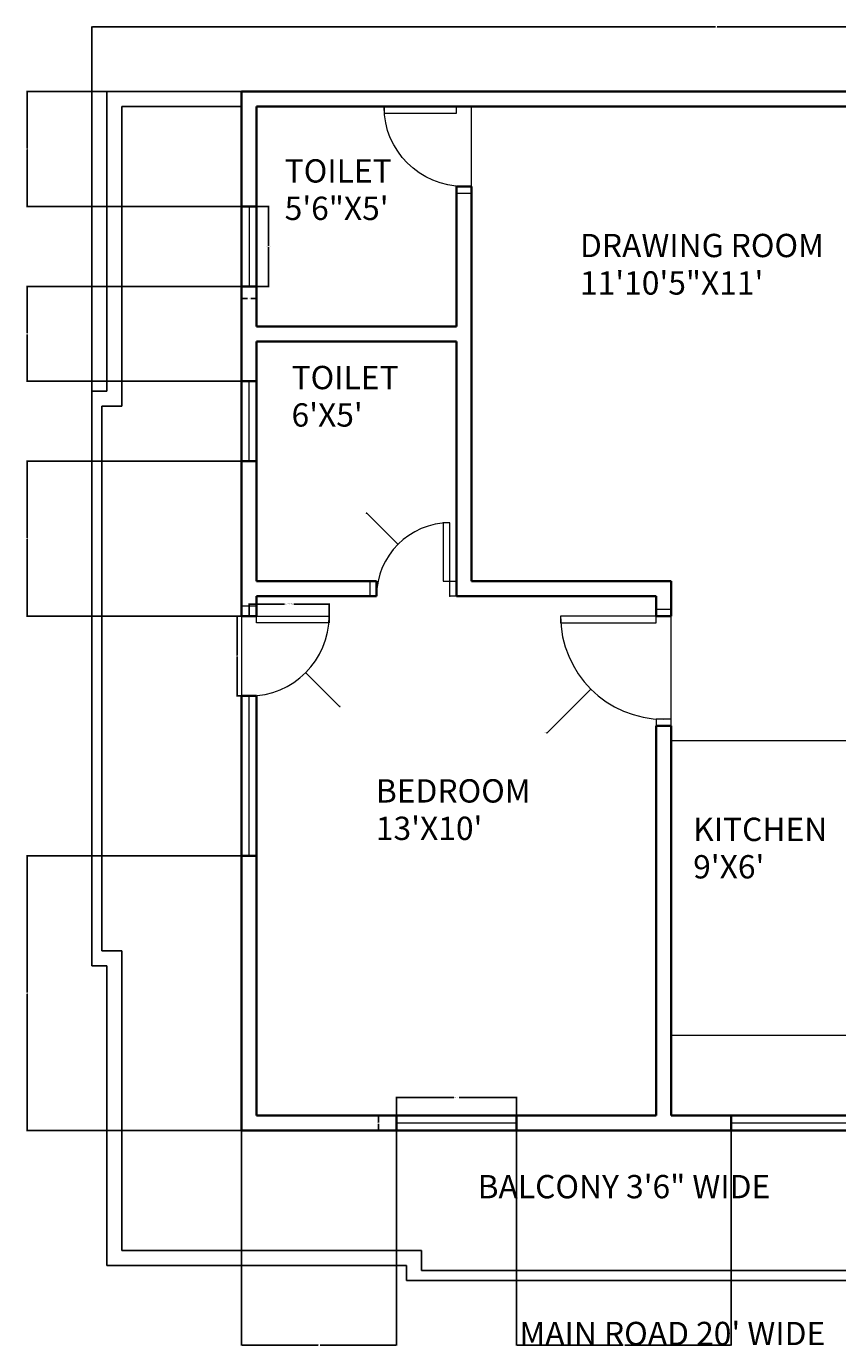
# Model space of a CAD drawing. Units: millimetres. Extents: x 2284 to 2706, y 1197 to 2041.
# Tile 1 of 3: x 2291 to 2535, y 1197 to 1593. Entities that reach past the tile are written whole.
import ezdxf

# ---------------------------------------------------------------- set-up
doc = ezdxf.new("R2010")
doc.units = ezdxf.units.MM
for name, color, linetype, lineweight in [('A-ANNO-DIMS', 2, 'Continuous', 18), ('A-ANNO-TEXT', 7, 'Continuous', 30), ('A-AREA-IDEN', 7, 'Continuous', 30), ('A-DOOR', 7, 'Continuous', 18), ('A-FLOR-FIXT', 6, 'Continuous', 18)]:
    doc.layers.add(name, color=color, linetype=linetype, lineweight=lineweight)
for name, color, linetype, lineweight, true_color in [('A-GLAZ', 219, 'Continuous', 18, 0x642165), ('A-WALL', 11, 'Continuous', 35, 0xf27172), ('A-WALL-PRPT', 143, 'Continuous', 25, 0x7aafdf)]:
    doc.layers.add(name, color=color, linetype=linetype, lineweight=lineweight, true_color=true_color)
doc.styles.get("Standard").update_dxf_attribs({"font": 'arial.ttf'})
doc.dimstyles.get("Standard").update_dxf_attribs({"dimtxt": 0.18, "dimasz": 0.18, "dimexe": 0.18, "dimexo": 0.0625, "dimgap": 0.09, "dimtad": 0, "dimtih": 1, "dimtoh": 1, "dimdec": 4, "dimzin": 0, "dimdsep": 46, "dimtxsty": 'Standard', "dimcen": 0.09, "dimadec": 0, "dimazin": 0, "dimtfac": 1, "dimtdec": 4, "dimtofl": 0, "dimtmove": 0, "dimatfit": 3, "dimfxl": 1, "dimtolj": 1, "dimtzin": 0, "dimarcsym": 0})

# ---------------------------------------------------------------- blocks, each defined once
blk = doc.blocks.new('WIN-24')
for p, q in [((4.5, 24), (0, 24)), ((0, 24), (0, 0)), ((4.5, 24), (2.25, 24)), ((2.25, 24), (2.25, 0)), ((4.5, 0), (4.5, 24)), ((0, 0), (4.5, 0))]:
    blk.add_line(p, q)
blk = doc.blocks.new('WIN-36')
for p, q in [((36, 4.5), (0, 4.5)), ((0, 4.5), (0, 0)), ((36, 0), (36, 4.5)), ((36, 2.25), (0, 2.25)), ((0, 0), (36, 0)), ((36, 0), (36, 2.25))]:
    blk.add_line(p, q)
blk = doc.blocks.new('WIN-48')
for p, q in [((4.5, 48), (0, 48)), ((0, 48), (0, 0)), ((2.25, 0), (2.25, 48)), ((4.5, 0), (4.5, 48)), ((0, 0), (4.5, 0)), ((0, 0), (2.25, 0))]:
    blk.add_line(p, q)
blk = doc.blocks.new('DOOR-SWING-24')
for p, q in [((2.25, 24), (24, 24)), ((24, 24), (24, 22)), ((24, 22), (2.25, 22))]:
    blk.add_line(p, q)
blk.add_arc((0, 24), 24, 270, 0)
blk = doc.blocks.new('*D11')
at = {"layer": 'A-ANNO-DIMS', "color": 0, "lineweight": -2, "transparency": 16777216}
for p, q in [((2360.52, 1538.8), (2364.23, 1538.8)), ((2364.05, 1538.62), (2364.05, 1526.98)), ((2364.05, 1514.98), (2364.05, 1526.62)), ((2360.52, 1514.8), (2364.23, 1514.8))]:
    blk.add_line(p, q, dxfattribs=at)
at = {"layer": 'A-ANNO-DIMS', "color": 0, "transparency": 16777216}
for points in [[(2364.02, 1538.62), (2364.08, 1538.62), (2364.05, 1538.8)], [(2364.02, 1514.98), (2364.08, 1514.98), (2364.05, 1514.8)]]:
    blk.add_solid(points, dxfattribs=at)
at = {"layer": 'Defpoints', "color": 0, "transparency": 16777216}
for p in [(2360.45, 1538.8), (2364.05, 1538.8), (2360.45, 1514.8)]:
    blk.add_point(p, dxfattribs=at)
at = {"layer": 'A-ANNO-DIMS', "color": 0, "transparency": 16777216, "insert": (2364.05, 1526.8), "char_height": 0.18, "attachment_point": 5}
blk.add_mtext('\\A1;W1 24 TYP.', dxfattribs=at)
blk = doc.blocks.new('*D12')
at = {"layer": 'A-ANNO-DIMS', "color": 0, "lineweight": -2, "transparency": 16777216}
for p, q in [((2355.95, 1514.74), (2355.95, 1511.02)), ((2360.45, 1514.74), (2360.45, 1511.02)), ((2356.13, 1511.2), (2357.75, 1511.2)), ((2360.27, 1511.2), (2358.66, 1511.2))]:
    blk.add_line(p, q, dxfattribs=at)
at = {"layer": 'A-ANNO-DIMS', "color": 0, "transparency": 16777216}
for points in [[(2356.13, 1511.23), (2356.13, 1511.17), (2355.95, 1511.2)], [(2360.27, 1511.23), (2360.27, 1511.17), (2360.45, 1511.2)]]:
    blk.add_solid(points, dxfattribs=at)
at = {"layer": 'Defpoints', "color": 0, "transparency": 16777216}
for p in [(2355.95, 1514.8), (2360.45, 1514.8), (2360.45, 1511.2)]:
    blk.add_point(p, dxfattribs=at)
at = {"layer": 'A-ANNO-DIMS', "color": 0, "transparency": 16777216, "insert": (2358.2, 1511.2), "char_height": 0.18, "attachment_point": 5}
blk.add_mtext('\\A1;5 TYP.', dxfattribs=at)
blk = doc.blocks.new('*D13')
at = {"layer": 'A-ANNO-DIMS', "color": 0, "lineweight": -2, "transparency": 16777216}
for p, q in [((2402.45, 1265.86), (2402.45, 1271.38)), ((2402.63, 1271.2), (2419.7, 1271.2)), ((2438.27, 1271.2), (2421.21, 1271.2)), ((2438.45, 1265.86), (2438.45, 1271.38))]:
    blk.add_line(p, q, dxfattribs=at)
at = {"layer": 'A-ANNO-DIMS', "color": 0, "transparency": 16777216}
for points in [[(2402.63, 1271.23), (2402.63, 1271.17), (2402.45, 1271.2)], [(2438.27, 1271.23), (2438.27, 1271.17), (2438.45, 1271.2)]]:
    blk.add_solid(points, dxfattribs=at)
at = {"layer": 'Defpoints', "color": 0, "transparency": 16777216}
for p in [(2438.45, 1271.2), (2402.45, 1265.8), (2438.45, 1265.8)]:
    blk.add_point(p, dxfattribs=at)
at = {"layer": 'A-ANNO-DIMS', "color": 0, "transparency": 16777216, "insert": (2420.45, 1271.2), "char_height": 0.18, "attachment_point": 5}
blk.add_mtext('\\A1;W2 36 TYP.', dxfattribs=at)
blk = doc.blocks.new('*D14')
at = {"layer": 'A-ANNO-DIMS', "color": 0, "lineweight": -2, "transparency": 16777216}
for p, q in [((2402.39, 1265.8), (2396.87, 1265.8)), ((2397.05, 1265.62), (2397.05, 1263.73)), ((2402.39, 1261.3), (2396.87, 1261.3)), ((2397.05, 1261.48), (2397.05, 1263.37))]:
    blk.add_line(p, q, dxfattribs=at)
at = {"layer": 'A-ANNO-DIMS', "color": 0, "transparency": 16777216}
for points in [[(2397.02, 1265.62), (2397.08, 1265.62), (2397.05, 1265.8)], [(2397.02, 1261.48), (2397.08, 1261.48), (2397.05, 1261.3)]]:
    blk.add_solid(points, dxfattribs=at)
at = {"layer": 'Defpoints', "color": 0, "transparency": 16777216}
for p in [(2397.05, 1265.8), (2402.45, 1265.8), (2402.45, 1261.3)]:
    blk.add_point(p, dxfattribs=at)
at = {"layer": 'A-ANNO-DIMS', "color": 0, "transparency": 16777216, "insert": (2397.05, 1263.55), "char_height": 0.18, "attachment_point": 5}
blk.add_mtext('\\A1;5 TYP.', dxfattribs=at)
blk = doc.blocks.new('*D17')
at = {"layer": 'A-ANNO-DIMS', "color": 0, "lineweight": -2, "transparency": 16777216}
for p, q in [((2358.2, 1415.86), (2358.2, 1419.58)), ((2358.38, 1419.4), (2368.8, 1419.4)), ((2382.02, 1419.4), (2371.61, 1419.4)), ((2382.2, 1415.86), (2382.2, 1419.58))]:
    blk.add_line(p, q, dxfattribs=at)
at = {"layer": 'A-ANNO-DIMS', "color": 0, "transparency": 16777216}
for points in [[(2358.38, 1419.43), (2358.38, 1419.37), (2358.2, 1419.4)], [(2382.02, 1419.43), (2382.02, 1419.37), (2382.2, 1419.4)]]:
    blk.add_solid(points, dxfattribs=at)
at = {"layer": 'Defpoints', "color": 0, "transparency": 16777216}
for p in [(2382.2, 1419.4), (2358.2, 1415.8), (2382.2, 1415.8)]:
    blk.add_point(p, dxfattribs=at)
at = {"layer": 'A-ANNO-DIMS', "color": 0, "transparency": 16777216, "insert": (2370.2, 1419.4), "char_height": 0.18, "attachment_point": 5}
blk.add_mtext('\\A1;SWING DOOR 24 TYP.', dxfattribs=at)
blk = doc.blocks.new('*D18')
at = {"layer": 'A-ANNO-DIMS', "color": 0, "lineweight": -2, "transparency": 16777216}
for p, q in [((2358.14, 1415.8), (2354.42, 1415.8)), ((2354.6, 1415.62), (2354.6, 1403.98)), ((2354.6, 1391.98), (2354.6, 1403.62)), ((2358.14, 1391.8), (2354.42, 1391.8))]:
    blk.add_line(p, q, dxfattribs=at)
at = {"layer": 'A-ANNO-DIMS', "color": 0, "transparency": 16777216}
for points in [[(2354.57, 1415.62), (2354.63, 1415.62), (2354.6, 1415.8)], [(2354.57, 1391.98), (2354.63, 1391.98), (2354.6, 1391.8)]]:
    blk.add_solid(points, dxfattribs=at)
at = {"layer": 'Defpoints', "color": 0, "transparency": 16777216}
for p in [(2354.6, 1415.8), (2358.2, 1415.8), (2358.2, 1391.8)]:
    blk.add_point(p, dxfattribs=at)
at = {"layer": 'A-ANNO-DIMS', "color": 0, "transparency": 16777216, "insert": (2354.6, 1403.8), "char_height": 0.18, "attachment_point": 5}
blk.add_mtext('\\A1;24 TYP.', dxfattribs=at)
blk = doc.blocks.new('*D28')
at = {"layer": 'A-ANNO-DIMS', "color": 0, "lineweight": -2, "transparency": 16777216}
for p, q in [((2310.95, 1483.36), (2310.95, 1592.88)), ((2311.13, 1592.7), (2498.17, 1592.7)), ((2685.77, 1592.7), (2498.74, 1592.7)), ((2685.95, 1573.36), (2685.95, 1592.88))]:
    blk.add_line(p, q, dxfattribs=at)
at = {"layer": 'A-ANNO-DIMS', "color": 0, "transparency": 16777216}
for points in [[(2311.13, 1592.73), (2311.13, 1592.67), (2310.95, 1592.7)], [(2685.77, 1592.73), (2685.77, 1592.67), (2685.95, 1592.7)]]:
    blk.add_solid(points, dxfattribs=at)
at = {"layer": 'Defpoints', "color": 0, "transparency": 16777216}
for p in [(2685.95, 1592.7), (2685.95, 1573.3), (2310.95, 1483.3)]:
    blk.add_point(p, dxfattribs=at)
at = {"layer": 'A-ANNO-DIMS', "color": 0, "transparency": 16777216, "insert": (2498.45, 1592.7), "char_height": 0.18, "attachment_point": 5}
blk.add_mtext('\\A1;375', dxfattribs=at)
blk = doc.blocks.new('*D30')
at = {"layer": 'A-ANNO-DIMS', "color": 0, "lineweight": -2, "transparency": 16777216}
for p, q in [((2355.89, 1573.3), (2291.37, 1573.3)), ((2291.55, 1573.12), (2291.55, 1556.23)), ((2291.55, 1538.98), (2291.55, 1555.87)), ((2355.89, 1538.8), (2291.37, 1538.8))]:
    blk.add_line(p, q, dxfattribs=at)
at = {"layer": 'A-ANNO-DIMS', "color": 0, "transparency": 16777216}
for points in [[(2291.52, 1573.12), (2291.58, 1573.12), (2291.55, 1573.3)], [(2291.52, 1538.98), (2291.58, 1538.98), (2291.55, 1538.8)]]:
    blk.add_solid(points, dxfattribs=at)
at = {"layer": 'Defpoints', "color": 0, "transparency": 16777216}
for p in [(2291.55, 1573.3), (2355.95, 1573.3), (2355.95, 1538.8)]:
    blk.add_point(p, dxfattribs=at)
at = {"layer": 'A-ANNO-DIMS', "color": 0, "transparency": 16777216, "insert": (2291.55, 1556.05), "char_height": 0.18, "attachment_point": 5}
blk.add_mtext('\\A1;34.5', dxfattribs=at)
blk = doc.blocks.new('*D31')
at = {"layer": 'A-ANNO-DIMS', "color": 0, "lineweight": -2, "transparency": 16777216}
for p, q in [((2355.89, 1514.8), (2291.37, 1514.8)), ((2291.55, 1514.62), (2291.55, 1500.73)), ((2291.55, 1486.48), (2291.55, 1500.37)), ((2355.89, 1486.3), (2291.37, 1486.3))]:
    blk.add_line(p, q, dxfattribs=at)
at = {"layer": 'A-ANNO-DIMS', "color": 0, "transparency": 16777216}
for points in [[(2291.52, 1514.62), (2291.58, 1514.62), (2291.55, 1514.8)], [(2291.52, 1486.48), (2291.58, 1486.48), (2291.55, 1486.3)]]:
    blk.add_solid(points, dxfattribs=at)
at = {"layer": 'Defpoints', "color": 0, "transparency": 16777216}
for p in [(2291.55, 1514.8), (2355.95, 1514.8), (2355.95, 1486.3)]:
    blk.add_point(p, dxfattribs=at)
at = {"layer": 'A-ANNO-DIMS', "color": 0, "transparency": 16777216, "insert": (2291.55, 1500.55), "char_height": 0.18, "attachment_point": 5}
blk.add_mtext('\\A1;28.5', dxfattribs=at)
blk = doc.blocks.new('*D32')
at = {"layer": 'A-ANNO-DIMS', "color": 0, "lineweight": -2, "transparency": 16777216}
for p, q in [((2355.89, 1462.3), (2291.37, 1462.3)), ((2291.55, 1462.12), (2291.55, 1439.23)), ((2291.55, 1415.98), (2291.55, 1438.87)), ((2355.89, 1415.8), (2291.37, 1415.8))]:
    blk.add_line(p, q, dxfattribs=at)
at = {"layer": 'A-ANNO-DIMS', "color": 0, "transparency": 16777216}
for points in [[(2291.52, 1462.12), (2291.58, 1462.12), (2291.55, 1462.3)], [(2291.52, 1415.98), (2291.58, 1415.98), (2291.55, 1415.8)]]:
    blk.add_solid(points, dxfattribs=at)
at = {"layer": 'Defpoints', "color": 0, "transparency": 16777216}
for p in [(2291.55, 1462.3), (2355.95, 1462.3), (2355.95, 1415.8)]:
    blk.add_point(p, dxfattribs=at)
at = {"layer": 'A-ANNO-DIMS', "color": 0, "transparency": 16777216, "insert": (2291.55, 1439.05), "char_height": 0.18, "attachment_point": 5}
blk.add_mtext('\\A1;46.5', dxfattribs=at)
blk = doc.blocks.new('*D33')
at = {"layer": 'A-ANNO-DIMS', "color": 0, "lineweight": -2, "transparency": 16777216}
for p, q in [((2355.89, 1343.8), (2291.37, 1343.8)), ((2291.55, 1343.62), (2291.55, 1302.73)), ((2291.55, 1261.48), (2291.55, 1302.37)), ((2355.89, 1261.3), (2291.37, 1261.3))]:
    blk.add_line(p, q, dxfattribs=at)
at = {"layer": 'A-ANNO-DIMS', "color": 0, "transparency": 16777216}
for points in [[(2291.52, 1343.62), (2291.58, 1343.62), (2291.55, 1343.8)], [(2291.52, 1261.48), (2291.58, 1261.48), (2291.55, 1261.3)]]:
    blk.add_solid(points, dxfattribs=at)
at = {"layer": 'Defpoints', "color": 0, "transparency": 16777216}
for p in [(2291.55, 1343.8), (2355.95, 1343.8), (2355.95, 1261.3)]:
    blk.add_point(p, dxfattribs=at)
at = {"layer": 'A-ANNO-DIMS', "color": 0, "transparency": 16777216, "insert": (2291.55, 1302.55), "char_height": 0.18, "attachment_point": 5}
blk.add_mtext('\\A1;82.5', dxfattribs=at)
blk = doc.blocks.new('*D34')
at = {"layer": 'A-ANNO-DIMS', "color": 0, "lineweight": -2, "transparency": 16777216}
for p, q in [((2355.95, 1261.24), (2355.95, 1196.72)), ((2402.45, 1261.24), (2402.45, 1196.72)), ((2356.13, 1196.9), (2378.88, 1196.9)), ((2402.27, 1196.9), (2379.53, 1196.9))]:
    blk.add_line(p, q, dxfattribs=at)
at = {"layer": 'A-ANNO-DIMS', "color": 0, "transparency": 16777216}
for points in [[(2356.13, 1196.93), (2356.13, 1196.87), (2355.95, 1196.9)], [(2402.27, 1196.93), (2402.27, 1196.87), (2402.45, 1196.9)]]:
    blk.add_solid(points, dxfattribs=at)
at = {"layer": 'Defpoints', "color": 0, "transparency": 16777216}
for p in [(2355.95, 1261.3), (2402.45, 1261.3), (2402.45, 1196.9)]:
    blk.add_point(p, dxfattribs=at)
at = {"layer": 'A-ANNO-DIMS', "color": 0, "transparency": 16777216, "insert": (2379.2, 1196.9), "char_height": 0.18, "attachment_point": 5}
blk.add_mtext('\\A1;46.5', dxfattribs=at)
blk = doc.blocks.new('*D35')
at = {"layer": 'A-ANNO-DIMS', "color": 0, "lineweight": -2, "transparency": 16777216}
for p, q in [((2438.45, 1261.24), (2438.45, 1196.72)), ((2502.95, 1261.24), (2502.95, 1196.72)), ((2438.63, 1196.9), (2470.38, 1196.9)), ((2502.77, 1196.9), (2471.03, 1196.9))]:
    blk.add_line(p, q, dxfattribs=at)
at = {"layer": 'A-ANNO-DIMS', "color": 0, "transparency": 16777216}
for points in [[(2438.63, 1196.93), (2438.63, 1196.87), (2438.45, 1196.9)], [(2502.77, 1196.93), (2502.77, 1196.87), (2502.95, 1196.9)]]:
    blk.add_solid(points, dxfattribs=at)
at = {"layer": 'Defpoints', "color": 0, "transparency": 16777216}
for p in [(2438.45, 1261.3), (2502.95, 1261.3), (2502.95, 1196.9)]:
    blk.add_point(p, dxfattribs=at)
at = {"layer": 'A-ANNO-DIMS', "color": 0, "transparency": 16777216, "insert": (2470.7, 1196.9), "char_height": 0.18, "attachment_point": 5}
blk.add_mtext('\\A1;64.5', dxfattribs=at)
blk = doc.blocks.new('*D38')
at = {"layer": 'A-ANNO-DIMS', "color": 0, "lineweight": -2, "transparency": 16777216}
for p, q in [((2482.61, 1415.8), (2482.79, 1415.8)), ((2482.7, 1415.71), (2482.7, 1415.89)), ((2447.63, 1380.73), (2460.66, 1393.75)), ((2447.45, 1380.73), (2447.63, 1380.73))]:
    blk.add_line(p, q, dxfattribs=at)
at = {"layer": 'A-ANNO-DIMS', "color": 0, "transparency": 16777216}
blk.add_solid([(2460.64, 1393.77), (2460.68, 1393.73), (2460.78, 1393.88)], dxfattribs=at)
at = {"layer": 'Defpoints', "color": 0, "transparency": 16777216}
for p in [(2482.7, 1415.8), (2460.78, 1393.88)]:
    blk.add_point(p, dxfattribs=at)
at = {"layer": 'A-ANNO-DIMS', "color": 0, "transparency": 16777216, "insert": (2447.16, 1380.73), "char_height": 0.18, "attachment_point": 5}
blk.add_mtext('\\A1;R31', dxfattribs=at)
blk = doc.blocks.new('*D42')
at = {"layer": 'A-ANNO-DIMS', "color": 0, "lineweight": -2, "transparency": 16777216}
for p, q in [((2358.11, 1415.8), (2358.29, 1415.8)), ((2358.2, 1415.71), (2358.2, 1415.89)), ((2385.36, 1388.65), (2375.3, 1398.7)), ((2385.54, 1388.65), (2385.36, 1388.65))]:
    blk.add_line(p, q, dxfattribs=at)
at = {"layer": 'A-ANNO-DIMS', "color": 0, "transparency": 16777216}
blk.add_solid([(2375.32, 1398.72), (2375.28, 1398.68), (2375.18, 1398.83)], dxfattribs=at)
at = {"layer": 'Defpoints', "color": 0, "transparency": 16777216}
for p in [(2358.2, 1415.8), (2375.18, 1398.83)]:
    blk.add_point(p, dxfattribs=at)
at = {"layer": 'A-ANNO-DIMS', "color": 0, "transparency": 16777216, "insert": (2385.84, 1388.65), "char_height": 0.18, "attachment_point": 5}
blk.add_mtext('\\A1;R24', dxfattribs=at)
blk = doc.blocks.new('*D43')
at = {"layer": 'A-ANNO-DIMS', "color": 0, "lineweight": -2, "transparency": 16777216}
for p, q in [((2393.38, 1446.69), (2393.56, 1446.69)), ((2393.56, 1446.69), (2402.77, 1437.48)), ((2418.36, 1421.8), (2418.54, 1421.8)), ((2418.45, 1421.71), (2418.45, 1421.89))]:
    blk.add_line(p, q, dxfattribs=at)
at = {"layer": 'A-ANNO-DIMS', "color": 0, "transparency": 16777216}
blk.add_solid([(2402.79, 1437.5), (2402.75, 1437.46), (2402.9, 1437.36)], dxfattribs=at)
at = {"layer": 'Defpoints', "color": 0, "transparency": 16777216}
for p in [(2402.9, 1437.36), (2418.45, 1421.8)]:
    blk.add_point(p, dxfattribs=at)
at = {"layer": 'A-ANNO-DIMS', "color": 0, "transparency": 16777216, "insert": (2393.08, 1446.69), "char_height": 0.18, "attachment_point": 5}
blk.add_mtext('\\A1;R22', dxfattribs=at)

msp = doc.modelspace()

# ---------------------------------------------------------------- linework, layer by layer
at = {"layer": 'A-DOOR'}
for p, q in [((2420.45, 1566.8), (2420.45, 1568.8)), ((2424.95, 1542.8), (2424.95, 1568.8)), ((2424.95, 1544.8), (2420.45, 1544.8)), ((2420.45, 1544.8), (2420.45, 1542.8)), ((2420.45, 1542.8), (2424.95, 1542.8)), ((2418.45, 1443.8), (2416.45, 1443.8)), ((2416.45, 1443.8), (2416.45, 1426.3)), ((2418.45, 1426.3), (2418.45, 1443.8)), ((2396.45, 1426.3), (2394.45, 1426.3)), ((2394.45, 1426.3), (2394.45, 1421.8)), ((2396.45, 1421.8), (2396.45, 1426.3)), ((2416.45, 1426.3), (2418.45, 1426.3)), ((2418.45, 1421.8), (2418.45, 1426.3)), ((2418.45, 1426.3), (2420.45, 1426.3)), ((2360.45, 1418.8), (2355.95, 1418.8)), ((2355.95, 1418.8), (2355.95, 1415.8)), ((2360.45, 1415.8), (2360.45, 1418.8)), ((2394.45, 1421.8), (2396.45, 1421.8)), ((2420.45, 1421.8), (2418.45, 1421.8)), ((2355.95, 1415.8), (2355.95, 1415.8)), ((2355.95, 1415.8), (2360.45, 1415.8)), ((2360.45, 1415.8), (2355.95, 1415.8)), ((2355.95, 1415.8), (2355.95, 1391.8)), ((2360.45, 1413.8), (2360.45, 1417.3)), ((2480.45, 1415.8), (2451.7, 1415.8)), ((2451.7, 1415.8), (2451.7, 1413.8)), ((2484.95, 1417.8), (2480.45, 1417.8)), ((2480.45, 1417.8), (2480.45, 1415.8)), ((2480.45, 1413.8), (2480.45, 1415.8)), ((2480.45, 1415.8), (2484.95, 1415.8)), ((2484.95, 1415.8), (2484.95, 1417.8)), ((2484.95, 1384.8), (2484.95, 1415.8)), ((2451.7, 1413.8), (2480.45, 1413.8)), ((2484.95, 1384.8), (2480.45, 1384.8)), ((2480.45, 1384.8), (2480.45, 1382.8)), ((2484.95, 1382.8), (2484.95, 1384.8))]:
    msp.add_line(p, q, dxfattribs=at)
for centre, radius, start, end in [((2418.45, 1421.8), 22, 90, 180), ((2482.7, 1415.8), 31, 180, 270)]:
    msp.add_arc(centre, radius, start, end, dxfattribs=at)
at = {"layer": 'A-FLOR-FIXT'}
for p, q in [((2538.95, 1378.3), (2484.95, 1378.3)), ((2538.95, 1289.8), (2484.95, 1289.8))]:
    msp.add_line(p, q, dxfattribs=at)
at = {"layer": 'A-GLAZ'}
for p, q in [((2355.95, 1514.8), (2355.95, 1538.8)), ((2355.95, 1486.3), (2355.95, 1462.3)), ((2360.45, 1391.8), (2360.45, 1343.8)), ((2420.45, 1265.8), (2402.45, 1265.8)), ((2520.95, 1265.8), (2502.95, 1265.8)), ((2402.45, 1261.3), (2438.45, 1261.3)), ((2502.95, 1261.3), (2538.95, 1261.3))]:
    msp.add_line(p, q, dxfattribs=at)
at = {"layer": 'A-WALL'}
for p, q in [((2355.95, 1573.3), (2685.95, 1573.3)), ((2355.95, 1573.3), (2360.45, 1573.3)), ((2685.95, 1573.3), (2355.95, 1573.3)), ((2355.95, 1573.3), (2355.95, 1538.8)), ((2355.95, 1415.8), (2355.95, 1573.3)), ((2360.45, 1568.8), (2420.45, 1568.8)), ((2360.45, 1502.8), (2360.45, 1568.8)), ((2360.45, 1538.8), (2360.45, 1568.8)), ((2360.45, 1568.8), (2556.95, 1568.8)), ((2424.95, 1568.8), (2420.45, 1568.8)), ((2424.95, 1568.8), (2556.95, 1568.8)), ((2420.45, 1544.8), (2420.45, 1502.8)), ((2424.95, 1544.8), (2420.45, 1544.8)), ((2424.95, 1544.8), (2420.45, 1544.8)), ((2420.45, 1544.8), (2420.45, 1502.8)), ((2424.95, 1426.3), (2424.95, 1544.8)), ((2424.95, 1426.3), (2424.95, 1544.8)), ((2355.95, 1538.8), (2360.45, 1538.8)), ((2355.95, 1538.8), (2360.45, 1538.8)), ((2360.45, 1514.8), (2355.95, 1514.8)), ((2360.45, 1514.8), (2355.95, 1514.8)), ((2355.95, 1514.8), (2355.95, 1486.3)), ((2360.45, 1502.8), (2360.45, 1514.8)), ((2360.45, 1502.8), (2360.45, 1514.8)), ((2420.45, 1502.8), (2360.45, 1502.8)), ((2420.45, 1502.8), (2360.45, 1502.8)), ((2360.45, 1498.3), (2420.45, 1498.3)), ((2360.45, 1426.3), (2360.45, 1498.3)), ((2360.45, 1498.3), (2360.45, 1486.3)), ((2360.45, 1486.3), (2360.45, 1498.3)), ((2360.45, 1498.3), (2420.45, 1498.3)), ((2420.45, 1498.3), (2420.45, 1426.3)), ((2420.45, 1498.3), (2420.45, 1421.8)), ((2360.45, 1486.3), (2355.95, 1486.3)), ((2355.95, 1486.3), (2360.45, 1486.3)), ((2355.95, 1462.3), (2360.45, 1462.3)), ((2360.45, 1462.3), (2355.95, 1462.3)), ((2355.95, 1462.3), (2355.95, 1415.8)), ((2360.45, 1426.3), (2360.45, 1462.3)), ((2396.45, 1426.3), (2360.45, 1426.3)), ((2396.45, 1426.3), (2360.45, 1426.3)), ((2396.45, 1421.8), (2396.45, 1426.3)), ((2396.45, 1421.8), (2396.45, 1426.3)), ((2420.45, 1426.3), (2420.45, 1421.8)), ((2484.95, 1426.3), (2424.95, 1426.3)), ((2484.95, 1426.3), (2424.95, 1426.3)), ((2484.95, 1415.8), (2484.95, 1426.3)), ((2484.95, 1415.8), (2484.95, 1426.3)), ((2360.45, 1421.8), (2396.45, 1421.8)), ((2360.45, 1421.8), (2360.45, 1415.8)), ((2360.45, 1415.8), (2360.45, 1421.8)), ((2360.45, 1421.8), (2396.45, 1421.8)), ((2360.45, 1415.8), (2360.45, 1421.8)), ((2420.45, 1421.8), (2480.45, 1421.8)), ((2420.45, 1421.8), (2480.45, 1421.8)), ((2480.45, 1421.8), (2480.45, 1415.8)), ((2480.45, 1421.8), (2480.45, 1415.8)), ((2480.45, 1421.8), (2480.45, 1415.8)), ((2360.45, 1415.8), (2355.95, 1415.8)), ((2355.95, 1415.8), (2360.45, 1415.8)), ((2480.45, 1415.8), (2484.95, 1415.8)), ((2480.45, 1415.8), (2484.95, 1415.8)), ((2355.95, 1261.3), (2355.95, 1391.8)), ((2355.95, 1391.8), (2360.45, 1391.8)), ((2360.45, 1265.8), (2360.45, 1391.8)), ((2484.95, 1382.8), (2480.45, 1382.8)), ((2484.95, 1382.8), (2480.45, 1382.8)), ((2480.45, 1382.8), (2480.45, 1265.8)), ((2480.45, 1382.8), (2480.45, 1265.8)), ((2484.95, 1373.8), (2484.95, 1382.8)), ((2484.95, 1378.3), (2484.95, 1382.8)), ((2484.95, 1265.8), (2484.95, 1382.8)), ((2484.95, 1373.8), (2484.95, 1377.8)), ((2484.95, 1265.8), (2484.95, 1373.8)), ((2360.45, 1343.8), (2355.95, 1343.8)), ((2360.45, 1343.8), (2355.95, 1343.8)), ((2355.95, 1343.8), (2355.95, 1261.3)), ((2360.45, 1265.8), (2360.45, 1343.8)), ((2480.45, 1265.8), (2360.45, 1265.8)), ((2402.45, 1265.8), (2360.45, 1265.8)), ((2402.45, 1265.8), (2402.45, 1261.3)), ((2402.45, 1261.3), (2402.45, 1265.8)), ((2438.45, 1261.3), (2438.45, 1265.8)), ((2480.45, 1265.8), (2438.45, 1265.8)), ((2438.45, 1265.8), (2438.45, 1261.3)), ((2556.95, 1265.8), (2484.95, 1265.8)), ((2502.95, 1265.8), (2484.95, 1265.8)), ((2502.95, 1265.8), (2502.95, 1261.3)), ((2355.95, 1261.3), (2402.45, 1261.3)), ((2561.45, 1261.3), (2355.95, 1261.3)), ((2438.45, 1261.3), (2502.95, 1261.3))]:
    msp.add_line(p, q, dxfattribs=at)
at = {"layer": 'A-WALL-PRPT'}
for p, q in [((2315.45, 1568.8), (2315.45, 1573.3)), ((2315.45, 1573.3), (2355.95, 1573.3)), ((2315.45, 1483.3), (2315.45, 1573.3)), ((2315.45, 1573.3), (2355.95, 1573.3)), ((2315.45, 1483.3), (2315.45, 1568.8)), ((2355.95, 1568.8), (2319.95, 1568.8)), ((2319.95, 1568.8), (2319.95, 1496.8)), ((2355.95, 1568.8), (2319.95, 1568.8)), ((2319.95, 1568.8), (2319.95, 1478.8)), ((2319.95, 1496.8), (2319.95, 1478.8)), ((2310.95, 1478.8), (2310.95, 1483.3)), ((2310.95, 1483.3), (2315.45, 1483.3)), ((2310.95, 1310.8), (2310.95, 1483.3)), ((2310.95, 1483.3), (2315.45, 1483.3)), ((2310.95, 1310.8), (2310.95, 1478.8)), ((2319.95, 1478.8), (2313.95, 1478.8)), ((2313.95, 1315.3), (2313.95, 1478.8)), ((2319.95, 1478.8), (2313.95, 1478.8)), ((2313.95, 1478.8), (2313.95, 1315.3)), ((2319.95, 1315.3), (2313.95, 1315.3)), ((2313.95, 1315.3), (2319.95, 1315.3)), ((2319.95, 1225.3), (2319.95, 1315.3)), ((2319.95, 1315.3), (2319.95, 1225.3)), ((2315.45, 1310.8), (2310.95, 1310.8)), ((2315.45, 1310.8), (2310.95, 1310.8)), ((2315.45, 1220.8), (2315.45, 1310.8)), ((2315.45, 1220.8), (2315.45, 1310.8)), ((2355.95, 1225.3), (2319.95, 1225.3)), ((2319.95, 1225.3), (2409.95, 1225.3)), ((2319.95, 1225.3), (2409.95, 1225.3)), ((2409.95, 1225.3), (2409.95, 1219.3)), ((2409.95, 1225.3), (2409.95, 1219.3)), ((2319.95, 1220.8), (2315.45, 1220.8)), ((2405.45, 1220.8), (2315.45, 1220.8)), ((2405.45, 1220.8), (2319.95, 1220.8)), ((2405.45, 1216.3), (2405.45, 1220.8)), ((2405.45, 1216.3), (2405.45, 1220.8)), ((2409.95, 1216.3), (2405.45, 1216.3)), ((2595.95, 1216.3), (2405.45, 1216.3)), ((2591.45, 1219.3), (2409.95, 1219.3)), ((2409.95, 1219.3), (2591.45, 1219.3)), ((2595.95, 1216.3), (2409.95, 1216.3))]:
    msp.add_line(p, q, dxfattribs=at)

# ---------------------------------------------------------------- block references
at = {"layer": 'A-DOOR', "extrusion": (0, 0, -1), "zscale": -1}
msp.add_blockref('DOOR-SWING-24', (-2422.7, 1544.8), dxfattribs=at)
at = {"layer": 'A-DOOR'}
msp.add_blockref('DOOR-SWING-24', (2358.2, 1391.8), dxfattribs=at)
at = {"layer": 'A-GLAZ'}
for name, p in [('WIN-24', (2355.95, 1514.8)), ('WIN-48', (2355.95, 1343.8)), ('WIN-36', (2402.45, 1261.3))]:
    msp.add_blockref(name, p, dxfattribs=at)
at = {"layer": 'A-GLAZ', "extrusion": (0, 0, -1), "zscale": -1, "rotation": 180}
for name, p in [('WIN-24', (-2355.95, 1486.3)), ('WIN-36', (-2502.95, 1265.8))]:
    msp.add_blockref(name, p, dxfattribs=at)

# ---------------------------------------------------------------- texts
at = {"layer": 'A-ANNO-TEXT'}
msp.add_text("MAIN ROAD 20' WIDE", height=7, dxfattribs=at).set_placement((2439.33, 1196.86))
at = {"layer": 'A-AREA-IDEN'}
for s, p in [('TOILET', (2368.86, 1545.98)), ('5\'6"X5\'', (2368.86, 1534.74)), ('DRAWING ROOM', (2457.53, 1523.58)), ('11\'10\'5"X11\'', (2457.53, 1512.33)), ('TOILET', (2370.93, 1483.93)), ("6'X5'", (2370.93, 1472.69)), ('BEDROOM', (2396.25, 1359.8)), ("13'X10'", (2396.25, 1348.56)), ('KITCHEN', (2491.51, 1348.25)), ("9'X6'", (2491.51, 1337.01)), ('BALCONY 3\'6" WIDE', (2426.8, 1240.96))]:
    msp.add_text(s, height=7, dxfattribs=at).set_placement(p)

# ---------------------------------------------------------------- dimensions: what is measured, and where the dimension line sits
at = {"layer": 'A-ANNO-DIMS'}
for base, p1, p2, override, picture, middle in [((2685.95, 1592.7), (2310.95, 1483.3), (2685.95, 1573.3), {"dimdec": 0, "dimlfac": 1, "dimrnd": 0, "dimzin": 0, "dimdsep": 46, "dimlunit": 2}, '*D28', (2498.45, 1592.7)), ((2402.45, 1196.9), (2355.95, 1261.3), (2402.45, 1261.3), {"dimdec": 1, "dimlfac": 1, "dimrnd": 0, "dimzin": 0, "dimdsep": 46, "dimlunit": 2}, '*D34', (2379.2, 1196.9)), ((2502.95, 1196.9), (2438.45, 1261.3), (2502.95, 1261.3), {"dimdec": 1, "dimlfac": 1, "dimrnd": 0, "dimzin": 0, "dimdsep": 46, "dimlunit": 2}, '*D35', (2470.7, 1196.9))]:
    dim = msp.add_linear_dim(base=base, p1=p1, p2=p2, dimstyle='Standard', override=override, dxfattribs=at)
    dim.commit()
    dim.dimension.update_dxf_attribs({"geometry": picture, "text_midpoint": middle})
for base, p1, p2, picture, middle in [((2291.55, 1573.3), (2355.95, 1538.8), (2355.95, 1573.3), '*D30', (2291.55, 1556.05)), ((2291.55, 1514.8), (2355.95, 1486.3), (2355.95, 1514.8), '*D31', (2291.55, 1500.55)), ((2291.55, 1462.3), (2355.95, 1415.8), (2355.95, 1462.3), '*D32', (2291.55, 1439.05)), ((2291.55, 1343.8), (2355.95, 1261.3), (2355.95, 1343.8), '*D33', (2291.55, 1302.55))]:
    dim = msp.add_linear_dim(base=base, p1=p1, p2=p2, angle=90, dimstyle='Standard', override={"dimdec": 1, "dimlfac": 1, "dimrnd": 0, "dimzin": 0, "dimdsep": 46, "dimlunit": 2}, dxfattribs=at)
    dim.commit()
    dim.dimension.update_dxf_attribs({"geometry": picture, "text_midpoint": middle})
for base, p1, p2, text, picture, middle in [((2364.05, 1538.8), (2360.45, 1514.8), (2360.45, 1538.8), 'W1 <> TYP.', '*D11', (2364.05, 1526.8)), ((2354.6, 1415.8), (2358.2, 1391.8), (2358.2, 1415.8), '<> TYP.', '*D18', (2354.6, 1403.8)), ((2397.05492415, 1265.80003665), (2402.45492415, 1261.30003665), (2402.45492415, 1265.80003665), '<> TYP.', '*D14', (2397.05492415, 1263.55003665))]:
    dim = msp.add_linear_dim(base=base, p1=p1, p2=p2, angle=90, text=text, dimstyle='Standard', override={"dimdec": 0, "dimlfac": 1, "dimrnd": 0, "dimzin": 0, "dimdsep": 46, "dimlunit": 2}, dxfattribs=at)
    dim.commit()
    dim.dimension.update_dxf_attribs({"geometry": picture, "text_midpoint": middle})
for base, p1, p2, text, picture, middle in [((2360.45492415, 1511.20003665), (2355.95492415, 1514.80003665), (2360.45492415, 1514.80003665), '<> TYP.', '*D12', (2358.20492415, 1511.20003665)), ((2382.2, 1419.4), (2358.2, 1415.8), (2382.2, 1415.8), 'SWING DOOR <> TYP.', '*D17', (2370.2, 1419.4)), ((2438.45, 1271.2), (2402.45, 1265.8), (2438.45, 1265.8), 'W2 <> TYP.', '*D13', (2420.45, 1271.2))]:
    dim = msp.add_linear_dim(base=base, p1=p1, p2=p2, text=text, dimstyle='Standard', override={"dimdec": 0, "dimlfac": 1, "dimrnd": 0, "dimzin": 0, "dimdsep": 46, "dimlunit": 2}, dxfattribs=at)
    dim.commit()
    dim.dimension.update_dxf_attribs({"geometry": picture, "text_midpoint": middle})
for center, mpoint, picture, middle in [((2418.45, 1421.8), (2402.9, 1437.36), '*D43', (2393.08, 1446.69)), ((2358.2, 1415.8), (2375.18, 1398.83), '*D42', (2385.84, 1388.65)), ((2482.7, 1415.8), (2460.78, 1393.88), '*D38', (2447.16, 1380.73))]:
    dim = msp.add_radius_dim(center=center, mpoint=mpoint, dimstyle='Standard', override={"dimdec": 0, "dimlfac": 1, "dimrnd": 0, "dimzin": 0, "dimdsep": 46, "dimlunit": 2}, dxfattribs=at)
    dim.commit()
    dim.dimension.update_dxf_attribs({"geometry": picture, "text_midpoint": middle, "dimtype": 164})

doc.saveas('drawing.dxf')
